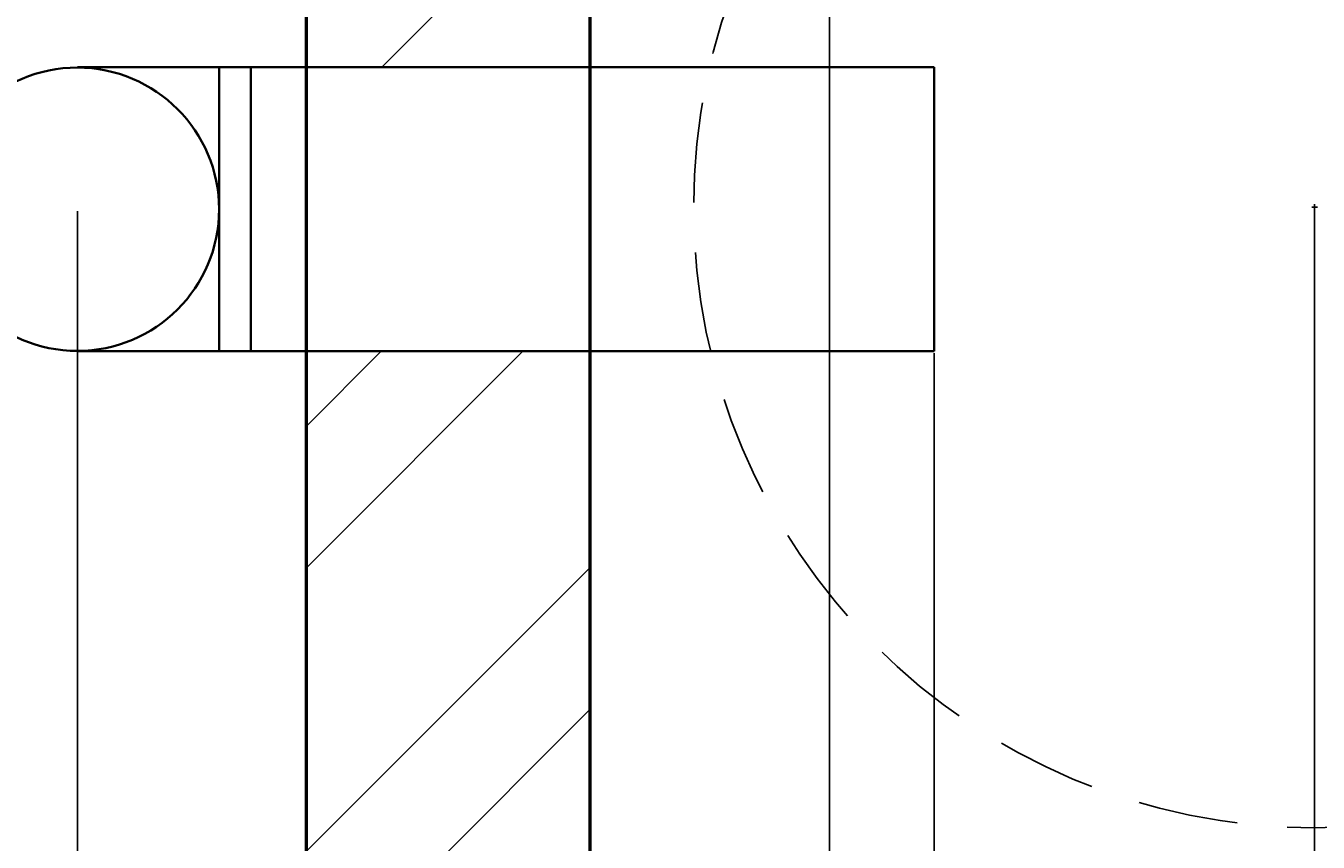
# Model space of a CAD drawing. Units: inches. Extents: x 2812 to 3051, y 1398 to 1659.
# Tile 59 of 65: x 2944 to 2984, y 1579 to 1605. Entities that reach past the tile are written whole.
import ezdxf

# ---------------------------------------------------------------- set-up
doc = ezdxf.new("R2010")
doc.units = ezdxf.units.IN
doc.linetypes.add('HIDDEN2', pattern=[4.7625, 3.175, -1.5875])
for name, color, linetype, lineweight in [('A-ANNO-DIMS', 2, 'Continuous', 18), ('P-SANR-PIPE', 4, 'Continuous', 35), ('S-CONC', 7, 'Continuous', 50), ('S-CONC-HIDN', 8, 'HIDDEN2', 25), ('S-CONC-PATT', 8, 'Continuous', 18)]:
    doc.layers.add(name, color=color, linetype=linetype, lineweight=lineweight)
doc.styles.get("Standard").update_dxf_attribs({"font": 'arial.ttf'})
doc.dimstyles.get("Standard").update_dxf_attribs({"dimtxt": 0.18, "dimasz": 0.18, "dimexe": 0.18, "dimexo": 0.0625, "dimgap": 0.09, "dimtad": 0, "dimtih": 1, "dimtoh": 1, "dimdec": 4, "dimzin": 0, "dimdsep": 46, "dimtxsty": 'Standard', "dimcen": 0.09, "dimadec": 0, "dimazin": 0, "dimtfac": 1, "dimtdec": 4, "dimtofl": 0, "dimtmove": 0, "dimatfit": 3, "dimfxl": 1, "dimtolj": 1, "dimtzin": 0, "dimarcsym": 0})

# ---------------------------------------------------------------- blocks, each defined once
blk = doc.blocks.new('*D30')
at = {"layer": 'A-ANNO-DIMS', "color": 0, "lineweight": -2, "transparency": 16777216}
for p, q in [((2945.147, 1598.692), (2945.147, 1397.505)), ((2952.385, 1559.757), (2952.385, 1397.505)), ((2945.327, 1397.685), (2948.373, 1397.685)), ((2952.205, 1397.685), (2949.159, 1397.685))]:
    blk.add_line(p, q, dxfattribs=at)
at = {"layer": 'A-ANNO-DIMS', "color": 0, "transparency": 16777216}
for points in [[(2945.327, 1397.715), (2945.327, 1397.655), (2945.147, 1397.685)], [(2952.205, 1397.715), (2952.205, 1397.655), (2952.385, 1397.685)]]:
    blk.add_solid(points, dxfattribs=at)
at = {"layer": 'Defpoints', "color": 0, "transparency": 16777216}
for p in [(2945.147, 1598.754), (2952.385, 1559.82), (2952.385, 1397.685)]:
    blk.add_point(p, dxfattribs=at)
at = {"layer": 'A-ANNO-DIMS', "color": 0, "transparency": 16777216, "insert": (2948.766, 1397.685), "char_height": 0.18, "attachment_point": 5}
blk.add_mtext('\\A1;7.238', dxfattribs=at)
blk = doc.blocks.new('*D31')
at = {"layer": 'A-ANNO-DIMS', "color": 0, "lineweight": -2, "transparency": 16777216}
for p, q in [((2972.272, 1594.192), (2972.272, 1397.505)), ((2961.385, 1559.757), (2961.385, 1397.505)), ((2961.565, 1397.685), (2966.373, 1397.685)), ((2972.092, 1397.685), (2967.283, 1397.685))]:
    blk.add_line(p, q, dxfattribs=at)
at = {"layer": 'A-ANNO-DIMS', "color": 0, "transparency": 16777216}
for points in [[(2961.565, 1397.715), (2961.565, 1397.655), (2961.385, 1397.685)], [(2972.092, 1397.715), (2972.092, 1397.655), (2972.272, 1397.685)]]:
    blk.add_solid(points, dxfattribs=at)
at = {"layer": 'Defpoints', "color": 0, "transparency": 16777216}
for p in [(2972.272, 1594.254), (2961.385, 1559.82), (2972.272, 1397.685)]:
    blk.add_point(p, dxfattribs=at)
at = {"layer": 'A-ANNO-DIMS', "color": 0, "transparency": 16777216, "insert": (2966.828, 1397.685), "char_height": 0.18, "attachment_point": 5}
blk.add_mtext('\\A1;10.887', dxfattribs=at)
blk = doc.blocks.new('*D32')
at = {"layer": 'A-ANNO-DIMS', "color": 0, "lineweight": -2, "transparency": 16777216}
for p, q in [((2984.316, 1598.757), (2984.316, 1397.505)), ((2972.272, 1594.192), (2972.272, 1397.505)), ((2972.452, 1397.685), (2977.839, 1397.685)), ((2984.136, 1397.685), (2978.748, 1397.685))]:
    blk.add_line(p, q, dxfattribs=at)
at = {"layer": 'A-ANNO-DIMS', "color": 0, "transparency": 16777216}
for points in [[(2972.452, 1397.715), (2972.452, 1397.655), (2972.272, 1397.685)], [(2984.136, 1397.715), (2984.136, 1397.655), (2984.316, 1397.685)]]:
    blk.add_solid(points, dxfattribs=at)
at = {"layer": 'Defpoints', "color": 0, "transparency": 16777216}
for p in [(2984.316, 1598.82), (2972.272, 1594.254), (2984.316, 1397.685)]:
    blk.add_point(p, dxfattribs=at)
at = {"layer": 'A-ANNO-DIMS', "color": 0, "transparency": 16777216, "insert": (2978.294, 1397.685), "char_height": 0.18, "attachment_point": 5}
blk.add_mtext('\\A1;12.044', dxfattribs=at)
blk = doc.blocks.new('*D69')
at = {"layer": 'A-ANNO-DIMS', "color": 0, "lineweight": -2, "transparency": 16777216}
for p, q in [((2961.385, 1472.098), (2961.385, 1659.35)), ((2961.565, 1659.17), (2964.795, 1659.17)), ((2968.776, 1659.17), (2965.546, 1659.17)), ((2968.956, 1467.81), (2968.956, 1659.35))]:
    blk.add_line(p, q, dxfattribs=at)
at = {"layer": 'A-ANNO-DIMS', "color": 0, "transparency": 16777216}
for points in [[(2961.565, 1659.2), (2961.565, 1659.14), (2961.385, 1659.17)], [(2968.776, 1659.2), (2968.776, 1659.14), (2968.956, 1659.17)]]:
    blk.add_solid(points, dxfattribs=at)
at = {"layer": 'Defpoints', "color": 0, "transparency": 16777216}
for p in [(2968.956, 1659.17), (2961.385, 1472.035), (2968.956, 1467.747)]:
    blk.add_point(p, dxfattribs=at)
at = {"layer": 'A-ANNO-DIMS', "color": 0, "transparency": 16777216, "insert": (2965.17, 1659.17), "char_height": 0.18, "attachment_point": 5}
blk.add_mtext('\\A1;7.571', dxfattribs=at)
blk = doc.blocks.new('*D83')
at = {"layer": 'A-ANNO-DIMS', "color": 0, "lineweight": -2, "transparency": 16777216}
for p, q in [((2984.316, 1598.73), (2984.316, 1598.91)), ((2984.226, 1598.82), (2984.406, 1598.82)), ((3015.77, 1598.82), (3004.154, 1598.82))]:
    blk.add_line(p, q, dxfattribs=at)
at = {"layer": 'A-ANNO-DIMS', "color": 0, "transparency": 16777216}
blk.add_solid([(3004.154, 1598.85), (3004.154, 1598.79), (3003.974, 1598.82)], dxfattribs=at)
at = {"layer": 'Defpoints', "color": 0, "transparency": 16777216}
for p in [(2964.657, 1598.82), (3003.974, 1598.82)]:
    blk.add_point(p, dxfattribs=at)
at = {"layer": 'A-ANNO-DIMS', "color": 0, "transparency": 16777216, "insert": (3016.26, 1598.82), "char_height": 0.18, "attachment_point": 5}
blk.add_mtext('\\A1;∅39.32', dxfattribs=at)

msp = doc.modelspace()

# ---------------------------------------------------------------- hatches: boundary and pattern name
at = {"layer": 'S-CONC-PATT'}
h = msp.add_hatch(dxfattribs=at)
h.set_pattern_fill('ANSI32', color=256)
h.paths.add_polyline_path([(2961.3849, 1637.82), (2952.3849, 1637.82), (2952.3849, 1603.2541), (2961.3849, 1603.2541)])
h.paths.add_polyline_path([(2961.3849, 1594.2541), (2952.3849, 1594.2541), (2952.3849, 1559.82), (2961.3849, 1559.82)])
h.paths.add_polyline_path([(2883.3849, 1637.82), (2880.3849, 1637.82), (2880.3849, 1559.82), (2883.3849, 1559.82)])

# ---------------------------------------------------------------- linework, layer by layer
at = {"layer": 'P-SANR-PIPE'}
for p, q in [((2945.1467, 1603.2541), (2972.2716, 1603.2541)), ((2949.6335, 1594.2541), (2949.6335, 1603.2541)), ((2949.6335, 1603.2541), (2950.6335, 1603.2541)), ((2950.6335, 1603.2541), (2950.6335, 1594.2541)), ((2972.2716, 1603.2541), (2972.2716, 1594.2541)), ((2949.6335, 1598.7541), (2949.6335, 1594.2541)), ((2972.2716, 1594.2541), (2945.1467, 1594.2541))]:
    msp.add_line(p, q, dxfattribs=at)
msp.add_circle((2945.1467, 1598.7541), 4.4867, dxfattribs=at)
at = {"layer": 'S-CONC'}
for p, q in [((2952.3849, 1637.82), (2952.3849, 1559.82)), ((2961.3849, 1559.82), (2961.3849, 1637.82))]:
    msp.add_line(p, q, dxfattribs=at)
at = {"layer": 'S-CONC-HIDN'}
msp.add_circle((2984.3156, 1598.82), 19.6588, dxfattribs=at)

# ---------------------------------------------------------------- dimensions: what is measured, and where the dimension line sits
at = {"layer": 'A-ANNO-DIMS'}
for base, p1, p2, picture, middle in [((2968.9558, 1659.17), (2961.3849, 1472.0354), (2968.9558, 1467.7474), '*D69', (2965.1704, 1659.17)), ((2952.3849, 1397.6854), (2945.1467, 1598.7541), (2952.3849, 1559.82), '*D30', (2948.7658, 1397.6854)), ((2984.3156, 1397.6854), (2972.2716, 1594.2541), (2984.3156, 1598.82), '*D32', (2978.2936, 1397.6854)), ((2972.2716, 1397.6854), (2961.3849, 1559.82), (2972.2716, 1594.2541), '*D31', (2966.8282, 1397.6854))]:
    dim = msp.add_linear_dim(base=base, p1=p1, p2=p2, dimstyle='Standard', override={"dimdec": 3, "dimlfac": 1, "dimrnd": 0, "dimzin": 0, "dimdsep": 46, "dimlunit": 2}, dxfattribs=at)
    dim.commit()
    dim.dimension.update_dxf_attribs({"geometry": picture, "text_midpoint": middle})
dim = msp.add_diameter_dim_2p(p1=(2964.6569, 1598.8199), p2=(3003.9744, 1598.82), dimstyle='Standard', override={"dimdec": 2, "dimlfac": 1, "dimrnd": 0, "dimzin": 0, "dimdsep": 46, "dimlunit": 2}, dxfattribs=at)
dim.commit()
dim.dimension.update_dxf_attribs({"geometry": '*D83', "text_midpoint": (3015.7697, 1598.82), "dimtype": 163})

doc.saveas('drawing.dxf')
